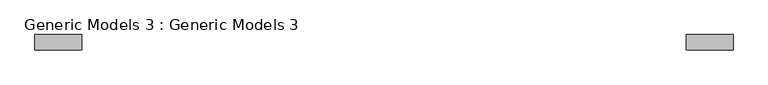
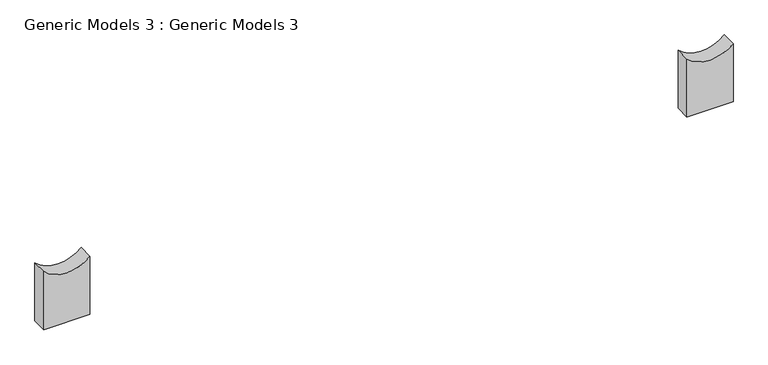
"""IFC4 building model written with IfcOpenShell, lengths in millimetres: proxy geometry, Generic Models 3 : Generic Models 3."""

from ifc_helpers import new_model, si_unit, point, frame, frame_2d, origin, place, context, project, spatial, polyline, circle_curve, trimmed, segment, composite_curve, outline, extrude, source, transform, mapped, element, save


def generic_models_3_generic_models_3_b11e1288(model_context):
    return source(origin(), model_context, "Body", "SweptSolid", [
        extrude(outline(composite_curve([segment(polyline([(9753.6, 5247.1584916), (9753.6, 6161.5584916), (10972.8, 6161.5584916)]), True, "CONTINUOUS"), segment(trimmed(circle_curve(frame_2d((11452.9762349, 5704.3584916)), 663.024175), [point((10972.8, 6161.5584916))], [point((10972.8, 5247.1584916))], True, "CARTESIAN"), True, "CONTINUOUS"), segment(polyline([(10972.8, 5247.1584916), (9753.6, 5247.1584916)]), True, "CONTINUOUS")], self_intersect=False)), frame((0.0, -8793.5477377, 0.0), z_axis=(0.0, 1.0, 0.0), x_axis=(0.0, 0.0, 1.0)), (0.0, 0.0, 1.0), 304.8),
        extrude(outline(composite_curve([segment(polyline([(9753.6, -7503.6415084), (9753.6, -6589.2415084), (10972.8, -6589.2415084)]), True, "CONTINUOUS"), segment(trimmed(circle_curve(frame_2d((11452.9762349, -7046.4415084)), 663.024175), [point((10972.8, -6589.2415084))], [point((10972.8, -7503.6415084))], True, "CARTESIAN"), True, "CONTINUOUS"), segment(polyline([(10972.8, -7503.6415084), (9753.6, -7503.6415084)]), True, "CONTINUOUS")], self_intersect=False)), frame((0.0, -8793.5477377, 0.0), z_axis=(0.0, 1.0, 0.0), x_axis=(0.0, 0.0, 1.0)), (0.0, 0.0, 1.0), 304.8),
    ])


if __name__ == "__main__":
    model = new_model("IFC4")
    model_context = context("Model", 3, world=origin())
    ifc_project = project(units=[si_unit("LENGTHUNIT", "METRE", prefix="MILLI")], contexts=[model_context])
    site = spatial("IfcSite", under=ifc_project)
    building = spatial("IfcBuilding", under=site)
    placement = place(None, origin())
    generic_models_3_generic_models_3_shape = generic_models_3_generic_models_3_b11e1288(model_context)
    element("IfcBuildingElementProxy", 1, Name="Generic Models 3 : Generic Models 3", ObjectType="Generic Models 3 : Generic Models 3", at=placement, inside=building, context=model_context, shape_type="MappedRepresentation", body=[
        mapped(generic_models_3_generic_models_3_shape, transform((0.0, 0.0, 0.0), x_axis=(1.0, 0.0, 0.0), y_axis=(0.0, 1.0, 0.0), z_axis=(0.0, 0.0, 1.0))),
    ])
    save(model, "model.ifc")

# Revit data of these elements
# Element 1 (IfcBuildingElementProxy, "Generic Models 3 : Generic Models 3")
#   Materials on its faces: "Door - Frame"
# Materials
#   "Door - Frame": colour RGB 118 70 51, transparency 0, Cost = 0
